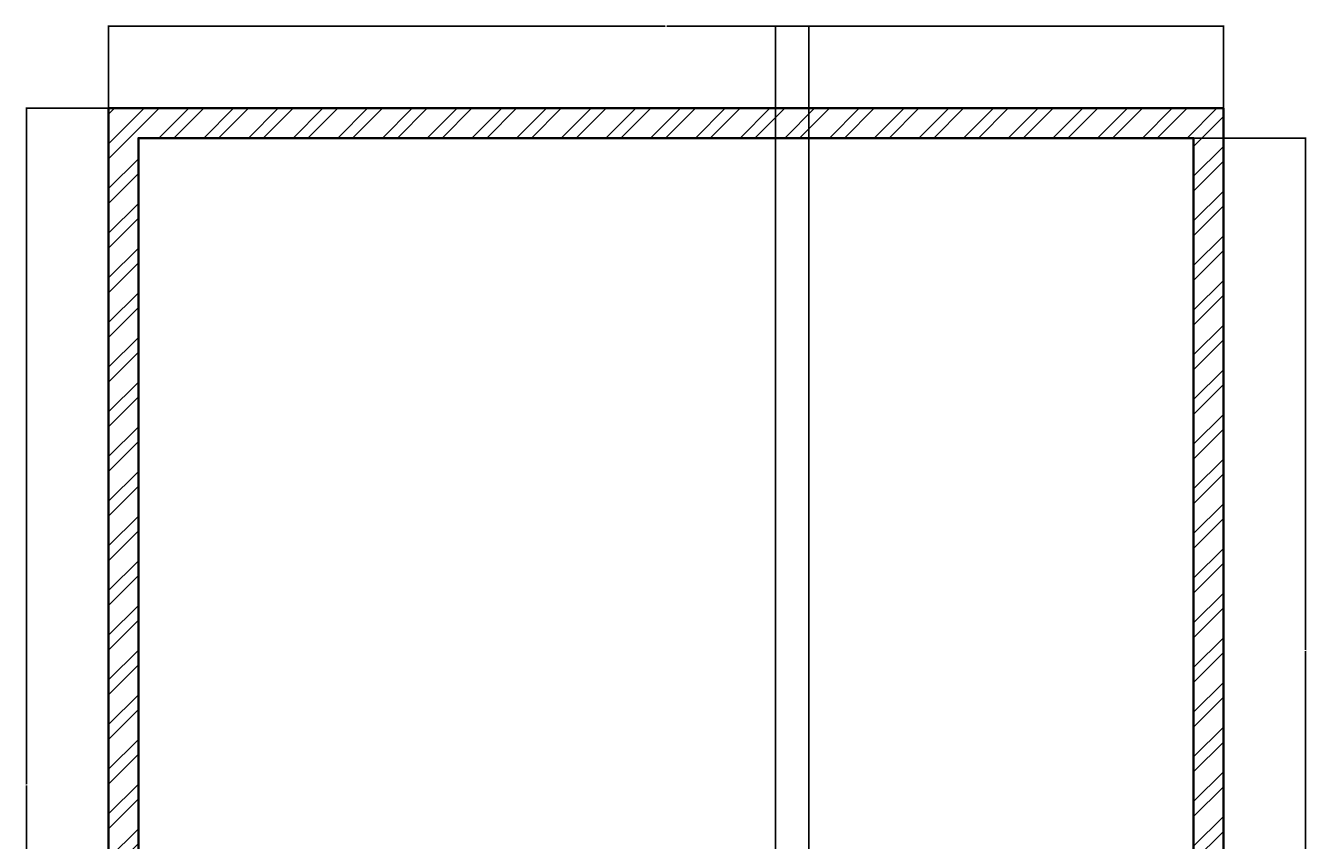
# Model space of a CAD drawing. Units: inches. Extents: x 2166 to 3588, y 1959 to 2628.
# Tile 13 of 13: x 3202 to 3588, y 2209 to 2455. Entities that reach past the tile are written whole.
import ezdxf

# ---------------------------------------------------------------- set-up
doc = ezdxf.new("R2010")
doc.units = ezdxf.units.IN
for name, color, linetype, lineweight in [('A-ANNO-DIMS', 2, 'Continuous', 18), ('A-WALL-PATT', 20, 'Continuous', 13), ('WALL', 40, 'Continuous', 35)]:
    doc.layers.add(name, color=color, linetype=linetype, lineweight=lineweight)
doc.styles.get("Standard").update_dxf_attribs({"font": 'arial.ttf'})
doc.dimstyles.get("Standard").update_dxf_attribs({"dimtxt": 0.18, "dimasz": 0.18, "dimexe": 0.18, "dimexo": 0.0625, "dimgap": 0.09, "dimtad": 0, "dimtih": 1, "dimtoh": 1, "dimdec": 4, "dimzin": 0, "dimdsep": 46, "dimtxsty": 'Standard', "dimcen": 0.09, "dimadec": 0, "dimazin": 0, "dimtfac": 1, "dimtdec": 4, "dimtofl": 0, "dimtmove": 0, "dimatfit": 3, "dimfxl": 1, "dimtolj": 1, "dimtzin": 0, "dimarcsym": 0})

# ---------------------------------------------------------------- blocks, each defined once
blk = doc.blocks.new('*D47')
at = {"layer": 'A-ANNO-DIMS', "color": 0, "lineweight": -2, "transparency": 16777216}
for p, q in [((3227.47, 2430.04), (3227.47, 2454.91)), ((3563.47, 2430.04), (3563.47, 2454.91)), ((3227.65, 2454.73), (3395.18, 2454.73)), ((3563.29, 2454.73), (3395.76, 2454.73))]:
    blk.add_line(p, q, dxfattribs=at)
at = {"layer": 'A-ANNO-DIMS', "color": 0, "transparency": 16777216}
for points in [[(3227.65, 2454.76), (3227.65, 2454.7), (3227.47, 2454.73)], [(3563.29, 2454.76), (3563.29, 2454.7), (3563.47, 2454.73)]]:
    blk.add_solid(points, dxfattribs=at)
at = {"layer": 'Defpoints', "color": 0, "transparency": 16777216}
for p in [(3563.47, 2454.73), (3227.47, 2429.98), (3563.47, 2429.98)]:
    blk.add_point(p, dxfattribs=at)
at = {"layer": 'A-ANNO-DIMS', "color": 0, "transparency": 16777216, "insert": (3395.47, 2454.73), "char_height": 0.18, "attachment_point": 5}
blk.add_mtext('\\A1;336', dxfattribs=at)
blk = doc.blocks.new('*D48')
at = {"layer": 'A-ANNO-DIMS', "color": 0, "lineweight": -2, "transparency": 16777216}
for p, q in [((3227.41, 2429.98), (3202.54, 2429.98)), ((3202.72, 2429.8), (3202.72, 2226.16)), ((3202.72, 2022.16), (3202.72, 2225.8)), ((3227.41, 2021.98), (3202.54, 2021.98))]:
    blk.add_line(p, q, dxfattribs=at)
at = {"layer": 'A-ANNO-DIMS', "color": 0, "transparency": 16777216}
for points in [[(3202.69, 2429.8), (3202.75, 2429.8), (3202.72, 2429.98)], [(3202.69, 2022.16), (3202.75, 2022.16), (3202.72, 2021.98)]]:
    blk.add_solid(points, dxfattribs=at)
at = {"layer": 'Defpoints', "color": 0, "transparency": 16777216}
for p in [(3202.72, 2429.98), (3227.47, 2429.98), (3227.47, 2021.98)]:
    blk.add_point(p, dxfattribs=at)
at = {"layer": 'A-ANNO-DIMS', "color": 0, "transparency": 16777216, "insert": (3202.72, 2225.98), "char_height": 0.18, "attachment_point": 5}
blk.add_mtext('\\A1;408', dxfattribs=at)
blk = doc.blocks.new('*D49')
at = {"layer": 'A-ANNO-DIMS', "color": 0, "lineweight": -2, "transparency": 16777216}
for p, q in [((3554.53, 2420.98), (3588.4, 2420.98)), ((3588.22, 2420.8), (3588.22, 2266.66)), ((3588.22, 2112.16), (3588.22, 2266.3)), ((3554.53, 2111.98), (3588.4, 2111.98))]:
    blk.add_line(p, q, dxfattribs=at)
at = {"layer": 'A-ANNO-DIMS', "color": 0, "transparency": 16777216}
for points in [[(3588.19, 2420.8), (3588.25, 2420.8), (3588.22, 2420.98)], [(3588.19, 2112.16), (3588.25, 2112.16), (3588.22, 2111.98)]]:
    blk.add_solid(points, dxfattribs=at)
at = {"layer": 'Defpoints', "color": 0, "transparency": 16777216}
for p in [(3554.47, 2420.98), (3588.22, 2420.98), (3554.47, 2111.98)]:
    blk.add_point(p, dxfattribs=at)
at = {"layer": 'A-ANNO-DIMS', "color": 0, "transparency": 16777216, "insert": (3588.22, 2266.48), "char_height": 0.18, "attachment_point": 5}
blk.add_mtext('\\A1;309', dxfattribs=at)
blk = doc.blocks.new('*D53')
at = {"layer": 'A-ANNO-DIMS', "color": 0, "lineweight": -2, "transparency": 16777216}
for p, q in [((3428.47, 2066.04), (3428.47, 2454.91)), ((3438.47, 2066.04), (3438.47, 2454.91)), ((3428.65, 2454.73), (3433.26, 2454.73)), ((3438.29, 2454.73), (3433.68, 2454.73))]:
    blk.add_line(p, q, dxfattribs=at)
at = {"layer": 'A-ANNO-DIMS', "color": 0, "transparency": 16777216}
for points in [[(3428.65, 2454.76), (3428.65, 2454.7), (3428.47, 2454.73)], [(3438.29, 2454.76), (3438.29, 2454.7), (3438.47, 2454.73)]]:
    blk.add_solid(points, dxfattribs=at)
at = {"layer": 'Defpoints', "color": 0, "transparency": 16777216}
for p in [(3438.47, 2454.73), (3428.47, 2065.98), (3438.47, 2065.98)]:
    blk.add_point(p, dxfattribs=at)
at = {"layer": 'A-ANNO-DIMS', "color": 0, "transparency": 16777216, "insert": (3433.47, 2454.73), "char_height": 0.18, "attachment_point": 5}
blk.add_mtext('\\A1;10', dxfattribs=at)

msp = doc.modelspace()

# ---------------------------------------------------------------- hatches: boundary and pattern name
at = {"layer": 'A-WALL-PATT'}
h = msp.add_hatch(dxfattribs=at)
h.set_pattern_fill('ANSI32', color=256)
h.paths.add_polyline_path([(3563.471, 2429.979), (3227.471, 2429.979), (3227.471, 2021.979), (3563.471, 2021.979)])
h.paths.add_polyline_path([(3236.471, 2420.979), (3554.471, 2420.979), (3554.471, 2111.979), (3236.471, 2111.979)], flags=16)
h.paths.add_polyline_path([(3236.471, 2102.979), (3554.471, 2102.979), (3554.471, 2030.979), (3236.471, 2030.979)], flags=16)
h.paths.add_polyline_path([(3518.471, 2085.283), (3518.471, 2067.979), (3458.471, 2067.979), (3458.471, 2085.283)], flags=0)
h.paths.add_polyline_path([(3434.656, 2082.283), (3442.194, 2082.283), (3442.194, 2087.514), (3434.656, 2087.514)], flags=8)
h.paths.add_polyline_path([(3522.671, 2094.512), (3521.752, 2052.984), (3545.541, 2052.457), (3546.46, 2093.986)], flags=8)

# ---------------------------------------------------------------- linework, layer by layer
at = {"layer": 'WALL'}
msp.add_lwpolyline([(3227.471, 2429.979), (3563.471, 2429.979), (3563.471, 2021.979), (3227.471, 2021.979)], close=True, dxfattribs=at)
msp.add_lwpolyline([(3236.471, 2111.979), (3236.471, 2420.979), (3554.471, 2420.979), (3554.471, 2111.979)], dxfattribs=at)

# ---------------------------------------------------------------- dimensions: what is measured, and where the dimension line sits
at = {"layer": 'A-ANNO-DIMS'}
for base, p1, p2, picture, middle in [((3563.471, 2454.729), (3227.471, 2429.979), (3563.471, 2429.979), '*D47', (3395.471, 2454.729)), ((3438.471, 2454.729), (3428.471, 2065.979), (3438.471, 2065.979), '*D53', (3433.471, 2454.729))]:
    dim = msp.add_linear_dim(base=base, p1=p1, p2=p2, dimstyle='Standard', override={"dimdec": 0, "dimlfac": 1, "dimrnd": 0, "dimzin": 0, "dimdsep": 46, "dimlunit": 2}, dxfattribs=at)
    dim.commit()
    dim.dimension.update_dxf_attribs({"geometry": picture, "text_midpoint": middle})
for base, p1, p2, picture, middle in [((3202.721, 2429.979), (3227.471, 2021.979), (3227.471, 2429.979), '*D48', (3202.721, 2225.979)), ((3588.221, 2420.979), (3554.471, 2111.979), (3554.471, 2420.979), '*D49', (3588.221, 2266.479))]:
    dim = msp.add_linear_dim(base=base, p1=p1, p2=p2, angle=90, dimstyle='Standard', override={"dimdec": 0, "dimlfac": 1, "dimrnd": 0, "dimzin": 0, "dimdsep": 46, "dimlunit": 2}, dxfattribs=at)
    dim.commit()
    dim.dimension.update_dxf_attribs({"geometry": picture, "text_midpoint": middle})

doc.saveas('drawing.dxf')
